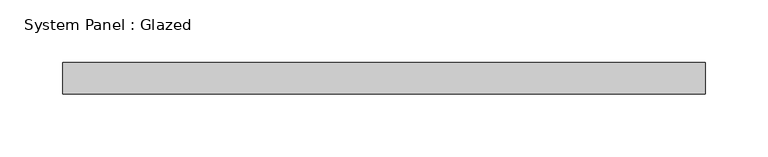
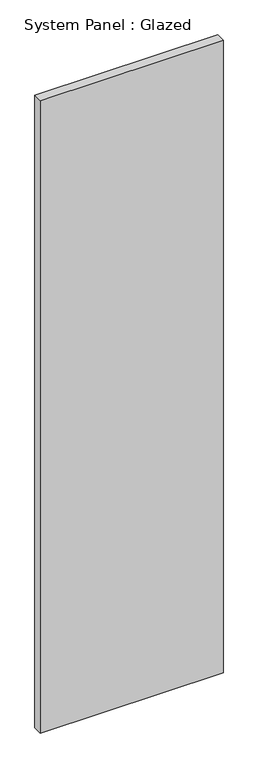
"""IFC4 building model written with IfcOpenShell, lengths in millimetres: plate geometry, System Panel : Glazed."""

from ifc_helpers import new_model, si_unit, origin, origin_with_axes, place, context, project, spatial, polyline, outline, extrude, source, transform, mapped, element, save


def system_panel_glazed_af17b7d9(model_context):
    return source(origin(), model_context, "Body", "SweptSolid", [
        extrude(outline(polyline([(257.175, 19.05), (-257.175, 19.05), (-257.175, 44.45), (257.175, 44.45), (257.175, 19.05)])), origin_with_axes(), (0.0, 0.0, 1.0), 1879.6),
    ])


if __name__ == "__main__":
    model = new_model("IFC4")
    model_context = context("Model", 3, world=origin())
    ifc_project = project(units=[si_unit("LENGTHUNIT", "METRE", prefix="MILLI")], contexts=[model_context])
    site = spatial("IfcSite", under=ifc_project)
    building = spatial("IfcBuilding", under=site)
    placement = place(None, origin())
    system_panel_glazed_shape = system_panel_glazed_af17b7d9(model_context)
    element("IfcPlate", 1, ObjectType="System Panel : Glazed", at=placement, inside=building, context=model_context, shape_type="MappedRepresentation", body=[
        mapped(system_panel_glazed_shape, transform((0.0, 0.0, 0.0), x_axis=(1.0, 0.0, 0.0), y_axis=(0.0, 1.0, 0.0), z_axis=(0.0, 0.0, 1.0))),
    ])
    save(model, "model.ifc")

# Revit data of these elements
# Type "System Panel : Glazed"
#   Construction Type Id = "GSP4R"
#   Analytic Construction = "1/8 in Pilkington single glazing"
#   Visual Light Transmittance = 0.9
#   Solar Heat Gain Coefficient = 0.86
#   Heat Transfer Coefficient (U) = 1.18115 BTU/(h·ft²·°F)
#   Define Thermal Properties by = 1
# Element 1 (IfcPlate, "System Panel : Glazed")
#   Materials on its faces: "Glass"
# Materials
#   "Glass": class "Glass", colour RGB 0 128 192, transparency 0.75, Description = "Soda Lime Glass", Cost = 0
